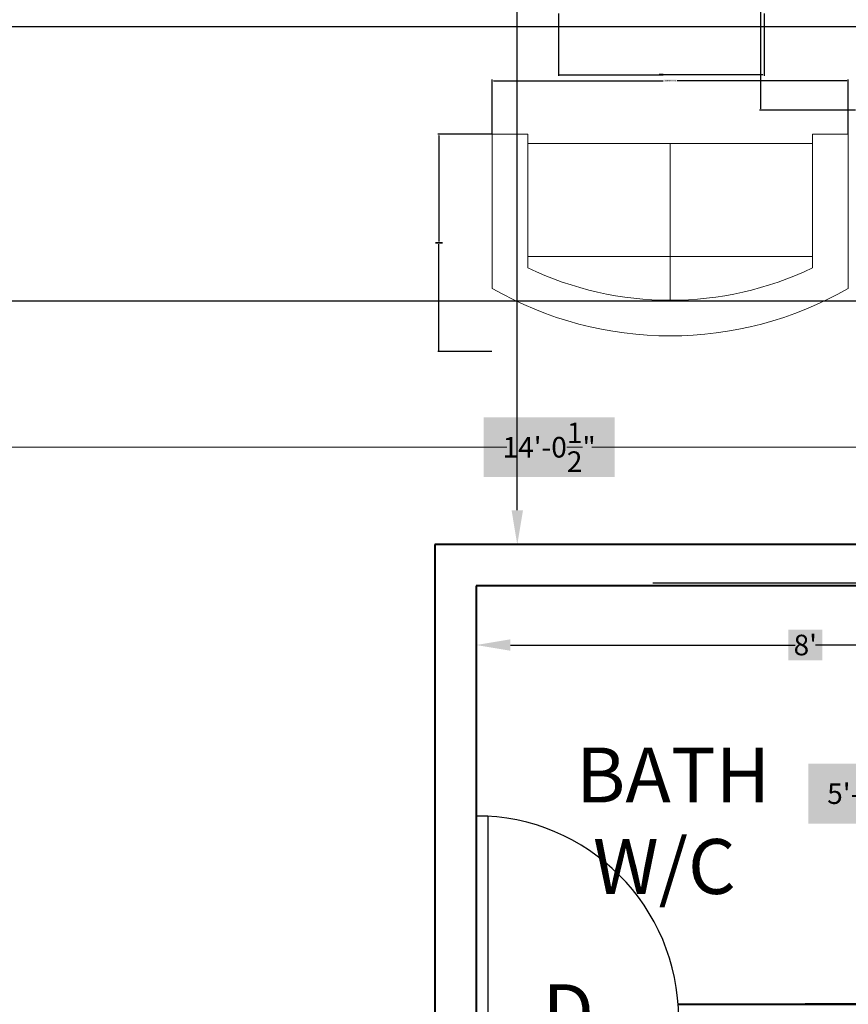
# Model space of a CAD drawing. Units: inches. Extents: x -301 to 715, y -607 to 364.
# Tile 97 of 141: x -39 to 82, y -77 to 67. Entities that reach past the tile are written whole.
import ezdxf

# ---------------------------------------------------------------- set-up
doc = ezdxf.new("R2010")
doc.units = ezdxf.units.IN
doc.header["$MEASUREMENT"] = 0
for name, color, linetype, lineweight in [('A-ANNO-DIMS', 2, 'Continuous', 18), ('A-ANNO-TEXT', 4, 'Continuous', 18), ('A-AREA-IDEN', 220, 'Continuous', 25), ('A-DOOR', 4, 'Continuous', 25), ('A-FURN', 8, 'Continuous', 18), ('A-WALL', 3, 'Continuous', 40)]:
    doc.layers.add(name, color=color, linetype=linetype, lineweight=lineweight)
doc.styles.get("Standard").update_dxf_attribs({"font": 'arial.ttf'})
doc.dimstyles.get("Standard").update_dxf_attribs({"dimtxt": 0.18, "dimasz": 0.18, "dimexe": 0.18, "dimexo": 0.0625, "dimgap": 0.09, "dimtad": 0, "dimtih": 1, "dimtoh": 1, "dimdec": 1, "dimzin": 0, "dimdsep": 46, "dimlunit": 4, "dimtxsty": 'Standard', "dimcen": 0.09, "dimclrd": 3, "dimclre": 4, "dimclrt": 6, "dimadec": 0, "dimazin": 0, "dimtfac": 1, "dimtdec": 1, "dimtofl": 0, "dimtmove": 0, "dimatfit": 3, "dimfxl": 1, "dimtfill": 2, "dimtfillclr": 51, "dimtolj": 1, "dimtzin": 0, "dimarcsym": 0})

# ---------------------------------------------------------------- blocks, each defined once
blk = doc.blocks.new('*U2')
for p, q in [((0, 0), (0, -100)), ((750, 0), (750, -100))]:
    blk.add_line(p, q)
blk.add_lwpolyline([(0, 0), (0, 750), (43.75, 750), (43.75, 0)], close=True)
blk.add_arc((0, 0), 750, 0, 90)
blk = doc.blocks.new('Sofa - Roundback Loveseat 5 ft.')
for p, q in [((0, -32.44198), (0, -5.99998)), ((-24, -33.99998), (-24, -11.46958)), ((24.00004, -33.99998), (24.00004, -11.46958)), ((-23.9998, -13.38178), (23.99986, -13.38178)), ((-24, -32.44198), (24.00004, -32.44198))]:
    blk.add_line(p, q)
for points in [[(-24, -33.99998), (-30, -33.99998), (-30, -7.99998)], [(30.00004, -7.99998), (30.00004, -33.99998), (24.00004, -33.99998)]]:
    blk.add_lwpolyline(points)
for centre, radius, start, end in [((0, -60.24998), 60.24998, 60.13715, 119.8628), ((0, -61.38438), 55.38444, 64.32083, 115.6792)]:
    blk.add_arc(centre, radius, start, end)
blk = doc.blocks.new('*D46')
at = {"layer": 'A-ANNO-DIMS', "color": 0, "lineweight": -2, "transparency": 16777216}
for p, q in [((27.9, -15.88), (27.9, -24.64)), ((123.9, -15.88), (123.9, -24.64)), ((32.9, -24.46), (74.42, -24.46)), ((118.9, -24.46), (77.37, -24.46))]:
    blk.add_line(p, q, dxfattribs=at)
at = {"layer": 'A-ANNO-DIMS', "color": 0, "transparency": 16777216}
for points in [[(32.9, -23.63), (32.9, -25.29), (27.9, -24.46)], [(118.9, -23.63), (118.9, -25.29), (123.9, -24.46)]]:
    blk.add_solid(points, dxfattribs=at)
at = {"layer": 'Defpoints', "color": 0, "transparency": 16777216}
for p in [(27.9, -15.82), (123.9, -15.82), (123.9, -24.46)]:
    blk.add_point(p, dxfattribs=at)
at = {"layer": 'A-ANNO-DIMS', "color": 0, "transparency": 16777216, "insert": (75.9, -24.46), "char_height": 3, "attachment_point": 5, "bg_fill": 1, "box_fill_scale": 1.25, "bg_fill_color": 51, "bg_fill_transparency": 0}
blk.add_mtext("\\A1;8'", dxfattribs=at)
blk = doc.blocks.new('*D47')
at = {"layer": 'A-ANNO-DIMS', "color": 0, "lineweight": -2, "transparency": 16777216}
for p, q in [((53.67, -15.42), (84.93, -15.42)), ((84.75, -20.42), (84.75, -42.49)), ((84.75, -71.82), (84.75, -49.75)), ((57.41, -76.82), (84.93, -76.82))]:
    blk.add_line(p, q, dxfattribs=at)
at = {"layer": 'A-ANNO-DIMS', "color": 0, "transparency": 16777216}
for points in [[(83.92, -20.42), (85.59, -20.42), (84.75, -15.42)], [(83.92, -71.82), (85.59, -71.82), (84.75, -76.82)]]:
    blk.add_solid(points, dxfattribs=at)
at = {"layer": 'Defpoints', "color": 0, "transparency": 16777216}
for p in [(53.6, -15.42), (84.75, -15.42), (57.35, -76.82)]:
    blk.add_point(p, dxfattribs=at)
at = {"layer": 'A-ANNO-DIMS', "color": 0, "transparency": 16777216, "insert": (84.75, -46.12), "char_height": 3, "attachment_point": 5, "bg_fill": 1, "box_fill_scale": 1.25, "bg_fill_color": 51, "bg_fill_transparency": 0}
blk.add_mtext('\\A1;5\'-1{\\H1x;\\S1/2;}"', dxfattribs=at)
blk = doc.blocks.new('*D48')
at = {"layer": 'A-ANNO-DIMS', "color": 0, "lineweight": -2, "transparency": 16777216}
for p, q in [((-45.6, -7.66), (-45.6, 4.54)), ((122.71, -8.55), (122.71, 4.54))]:
    blk.add_line(p, q, dxfattribs=at)
at = {"layer": 'A-ANNO-DIMS', "color": 0, "lineweight": 0, "transparency": 16777216}
for p, q in [((-40.6, 4.36), (32.36, 4.36)), ((117.71, 4.36), (44.75, 4.36))]:
    blk.add_line(p, q, dxfattribs=at)
at = {"layer": 'A-ANNO-DIMS', "color": 0, "transparency": 16777216}
for points in [[(-40.6, 5.2), (-40.6, 3.53), (-45.6, 4.36)], [(117.71, 5.2), (117.71, 3.53), (122.71, 4.36)]]:
    blk.add_solid(points, dxfattribs=at)
at = {"layer": 'Defpoints', "color": 0, "transparency": 16777216}
for p in [(-45.6, 4.36), (-45.6, -7.72), (122.71, -8.61)]:
    blk.add_point(p, dxfattribs=at)
at = {"layer": 'A-ANNO-DIMS', "color": 0, "transparency": 16777216, "insert": (38.55, 4.36), "char_height": 3, "attachment_point": 5, "bg_fill": 1, "box_fill_scale": 1.25, "bg_fill_color": 51, "bg_fill_transparency": 0}
blk.add_mtext('\\A1;14\'-0{\\H1x;\\S1/2;}"', dxfattribs=at)
blk = doc.blocks.new('*D49')
at = {"layer": 'A-ANNO-DIMS', "color": 0, "lineweight": -2, "transparency": 16777216}
for p, q in [((15.96, 193.18), (34.08, 193.18)), ((33.9, 188.18), (33.9, 93.3)), ((33.9, -4.82), (33.9, 90.06)), ((21.96, -9.82), (34.08, -9.82))]:
    blk.add_line(p, q, dxfattribs=at)
at = {"layer": 'A-ANNO-DIMS', "color": 0, "transparency": 16777216}
for points in [[(33.07, 188.18), (34.74, 188.18), (33.9, 193.18)], [(33.07, -4.82), (34.74, -4.82), (33.9, -9.82)]]:
    blk.add_solid(points, dxfattribs=at)
at = {"layer": 'Defpoints', "color": 0, "transparency": 16777216}
for p in [(15.9, 193.18), (33.9, 193.18), (21.9, -9.82)]:
    blk.add_point(p, dxfattribs=at)
at = {"layer": 'A-ANNO-DIMS', "color": 0, "transparency": 16777216, "insert": (33.9, 91.68), "char_height": 3, "attachment_point": 5, "bg_fill": 1, "box_fill_scale": 1.25, "bg_fill_color": 51, "bg_fill_transparency": 0}
blk.add_mtext('\\A1;16\'-11"', dxfattribs=at)
blk = doc.blocks.new('*D131')
at = {"layer": 'A-ANNO-DIMS', "color": 4, "lineweight": -2, "transparency": 16777216}
for p, q in [((39.9, 67.59), (39.9, 58.47)), ((69.9, 67.59), (69.9, 58.47))]:
    blk.add_line(p, q, dxfattribs=at)
at = {"layer": 'A-ANNO-DIMS', "color": 3, "lineweight": -2, "transparency": 16777216}
for p, q in [((40.08, 58.65), (54.57, 58.65)), ((69.72, 58.65), (55.23, 58.65))]:
    blk.add_line(p, q, dxfattribs=at)
at = {"layer": 'A-ANNO-DIMS', "color": 3, "transparency": 16777216}
for points in [[(40.08, 58.68), (40.08, 58.62), (39.9, 58.65)], [(69.72, 58.68), (69.72, 58.62), (69.9, 58.65)]]:
    blk.add_solid(points, dxfattribs=at)
at = {"layer": 'Defpoints', "color": 0, "transparency": 16777216}
for p in [(39.9, 67.65), (69.9, 67.65), (39.9, 58.65)]:
    blk.add_point(p, dxfattribs=at)
at = {"layer": 'A-ANNO-DIMS', "color": 6, "transparency": 16777216, "insert": (54.9, 58.65), "char_height": 0.18, "attachment_point": 5, "bg_fill": 1, "box_fill_scale": 1.25, "bg_fill_color": 51, "bg_fill_transparency": 0}
blk.add_mtext('\\A1;2\'-6"', dxfattribs=at)
blk = doc.blocks.new('*D132')
at = {"layer": 'A-ANNO-DIMS', "color": 4, "lineweight": -2, "transparency": 16777216}
for p, q in [((83.22, 145.95), (69.24, 145.95)), ((83.22, 53.5), (69.24, 53.5))]:
    blk.add_line(p, q, dxfattribs=at)
at = {"layer": 'A-ANNO-DIMS', "color": 3, "lineweight": -2, "transparency": 16777216}
for p, q in [((69.42, 145.77), (69.42, 99.91)), ((69.42, 53.68), (69.42, 99.55))]:
    blk.add_line(p, q, dxfattribs=at)
at = {"layer": 'A-ANNO-DIMS', "color": 3, "transparency": 16777216}
for points in [[(69.39, 145.77), (69.45, 145.77), (69.42, 145.95)], [(69.39, 53.68), (69.45, 53.68), (69.42, 53.5)]]:
    blk.add_solid(points, dxfattribs=at)
at = {"layer": 'Defpoints', "color": 0, "transparency": 16777216}
for p in [(83.29, 145.95), (69.42, 53.5), (83.29, 53.5)]:
    blk.add_point(p, dxfattribs=at)
at = {"layer": 'A-ANNO-DIMS', "color": 6, "transparency": 16777216, "insert": (69.42, 99.73), "char_height": 0.18, "attachment_point": 5, "bg_fill": 1, "box_fill_scale": 1.25, "bg_fill_color": 51, "bg_fill_transparency": 0}
blk.add_mtext('\\A1;SOFA 7\'-8 1/2"', dxfattribs=at)
blk = doc.blocks.new('*D134')
at = {"layer": 'A-ANNO-DIMS', "color": 4, "lineweight": -2, "transparency": 16777216}
for p, q in [((30.26, 50.05), (30.26, 57.95)), ((82.14, 50.05), (82.14, 57.95))]:
    blk.add_line(p, q, dxfattribs=at)
at = {"layer": 'A-ANNO-DIMS', "color": 3, "lineweight": -2, "transparency": 16777216}
for p, q in [((30.44, 57.77), (55.18, 57.77)), ((81.96, 57.77), (57.22, 57.77))]:
    blk.add_line(p, q, dxfattribs=at)
at = {"layer": 'A-ANNO-DIMS', "color": 3, "transparency": 16777216}
for points in [[(30.44, 57.8), (30.44, 57.74), (30.26, 57.77)], [(81.96, 57.8), (81.96, 57.74), (82.14, 57.77)]]:
    blk.add_solid(points, dxfattribs=at)
at = {"layer": 'Defpoints', "color": 0, "transparency": 16777216}
for p in [(30.26, 57.77), (30.26, 49.99), (82.14, 49.99)]:
    blk.add_point(p, dxfattribs=at)
at = {"layer": 'A-ANNO-DIMS', "color": 6, "transparency": 16777216, "insert": (56.2, 57.77), "char_height": 0.18, "attachment_point": 5, "bg_fill": 1, "box_fill_scale": 1.25, "bg_fill_color": 51, "bg_fill_transparency": 0}
blk.add_mtext('\\A1;LOVESEAT 4\'-4"', dxfattribs=at)
blk = doc.blocks.new('*D135')
at = {"layer": 'A-ANNO-DIMS', "color": 4, "lineweight": -2, "transparency": 16777216}
for p, q in [((30.2, 49.99), (22.3, 49.99)), ((30.2, 18.29), (22.3, 18.29))]:
    blk.add_line(p, q, dxfattribs=at)
at = {"layer": 'A-ANNO-DIMS', "color": 3, "lineweight": -2, "transparency": 16777216}
for p, q in [((22.48, 49.81), (22.48, 34.32)), ((22.48, 18.47), (22.48, 33.96))]:
    blk.add_line(p, q, dxfattribs=at)
at = {"layer": 'A-ANNO-DIMS', "color": 3, "transparency": 16777216}
for points in [[(22.45, 49.81), (22.51, 49.81), (22.48, 49.99)], [(22.45, 18.47), (22.51, 18.47), (22.48, 18.29)]]:
    blk.add_solid(points, dxfattribs=at)
at = {"layer": 'Defpoints', "color": 0, "transparency": 16777216}
for p in [(30.26, 49.99), (22.48, 18.29), (30.26, 18.29)]:
    blk.add_point(p, dxfattribs=at)
at = {"layer": 'A-ANNO-DIMS', "color": 6, "transparency": 16777216, "insert": (22.48, 34.14), "char_height": 0.18, "attachment_point": 5, "bg_fill": 1, "box_fill_scale": 1.25, "bg_fill_color": 51, "bg_fill_transparency": 0}
blk.add_mtext('\\A1;2\'-7 1/2"', dxfattribs=at)
blk = doc.blocks.new('*D149')
at = {"layer": 'A-ANNO-DIMS', "color": 4, "lineweight": -2, "transparency": 16777216}
for p, q in [((-51.54, 65.68), (233.66, 65.68)), ((-51.54, 25.68), (233.66, 25.68))]:
    blk.add_line(p, q, dxfattribs=at)
at = {"layer": 'A-ANNO-DIMS', "color": 3, "lineweight": -2, "transparency": 16777216}
for p, q in [((233.48, 65.5), (233.48, 45.86)), ((233.48, 25.86), (233.48, 45.5))]:
    blk.add_line(p, q, dxfattribs=at)
at = {"layer": 'A-ANNO-DIMS', "color": 3, "transparency": 16777216}
for points in [[(233.45, 65.5), (233.51, 65.5), (233.48, 65.68)], [(233.45, 25.86), (233.51, 25.86), (233.48, 25.68)]]:
    blk.add_solid(points, dxfattribs=at)
at = {"layer": 'Defpoints', "color": 0, "transparency": 16777216}
for p in [(-51.6, 65.68), (-51.6, 25.68), (233.48, 25.68)]:
    blk.add_point(p, dxfattribs=at)
at = {"layer": 'A-ANNO-DIMS', "color": 6, "transparency": 16777216, "insert": (233.48, 45.68), "char_height": 0.18, "attachment_point": 5, "bg_fill": 1, "box_fill_scale": 1.25, "bg_fill_color": 51, "bg_fill_transparency": 0}
blk.add_mtext('\\A1;3\'-4"', dxfattribs=at)

msp = doc.modelspace()

# ---------------------------------------------------------------- linework, layer by layer
at = {"layer": 'A-WALL'}
for p, q in [((21.9, -9.82), (21.9, -82.82)), ((123.9, -9.82), (21.9, -9.82)), ((123.9, -15.82), (27.9, -15.82)), ((27.9, -15.82), (27.9, -82.82)), ((57.35, -76.82), (123.9, -76.82)), ((123.9, -76.82), (75.9, -76.82))]:
    msp.add_line(p, q, dxfattribs=at)

# ---------------------------------------------------------------- block references
at = {"layer": 'A-DOOR', "xscale": 0.0393700787401575, "yscale": 0.0393700787401575, "zscale": 0.0393700787401575}
msp.add_blockref('*U2', (27.9, -78.88), dxfattribs=at)
at = {"layer": 'A-FURN', "xscale": 0.8646946346220261, "yscale": 0.8646946346220261, "zscale": 0.8646946346220261, "rotation": 180}
msp.add_blockref('Sofa - Roundback Loveseat 5 ft.', (56.2, 20.59), dxfattribs=at)

# ---------------------------------------------------------------- texts
at = {"layer": 'A-ANNO-TEXT'}
msp.add_text('D', height=8, dxfattribs=at).set_placement((37.58, -81.89))
at = {"layer": 'A-AREA-IDEN', "insert": (42.49, -39.4), "char_height": 8, "attachment_point": 1}
msp.add_mtext_dynamic_manual_height_columns('BATH\\P W/C', width=73.06, gutter_width=1, heights=[0], dxfattribs=at)

# ---------------------------------------------------------------- dimensions: what is measured, and where the dimension line sits
at = {"layer": 'A-ANNO-DIMS'}
for base, p1, p2, angle, override, picture, middle in [((33.9, 193.18), (21.9, -9.82), (15.9, 193.18), 90, {"dimtxt": 3, "dimasz": 5, "dimclrd": 0, "dimclre": 0, "dimclrt": 0}, '*D49', (33.9, 91.68)), ((39.9, 58.65), (69.9, 67.65), (39.9, 67.65), 180, {"dimdec": 1, "dimlfac": 1, "dimrnd": 0, "dimzin": 1, "dimdsep": 46, "dimlunit": 4, "dimfrac": 2}, '*D131', (54.9, 58.65)), ((233.48, 25.68), (-51.6, 65.68), (-51.6, 25.68), 90, {"dimdec": 1, "dimlfac": 1, "dimrnd": 0, "dimzin": 1, "dimdsep": 46, "dimlunit": 4, "dimfrac": 2}, '*D149', (233.48, 45.68)), ((22.48, 18.29), (30.26, 49.99), (30.26, 18.29), 270, {"dimdec": 1, "dimlfac": 1, "dimrnd": 0, "dimzin": 1, "dimdsep": 46, "dimlunit": 4, "dimfrac": 2}, '*D135', (22.48, 34.14)), ((84.75, -15.42), (57.35, -76.82), (53.6, -15.42), 90, {"dimtxt": 3, "dimasz": 5, "dimclrd": 0, "dimclre": 0, "dimclrt": 0}, '*D47', (84.75, -46.12))]:
    dim = msp.add_linear_dim(base=base, p1=p1, p2=p2, angle=angle, dimstyle='Standard', override=override, dxfattribs=at)
    dim.commit()
    dim.dimension.update_dxf_attribs({"geometry": picture, "text_midpoint": middle})
for base, p1, p2, angle, text, picture, middle in [((69.4192, 53.5044), (83.2867, 145.9543), (83.2867, 53.5044), 270, 'SOFA <>', '*D132', (69.4192, 99.7293)), ((30.26, 57.77), (82.14, 49.99), (30.26, 49.99), 180, 'LOVESEAT <>', '*D134', (56.2, 57.77))]:
    dim = msp.add_linear_dim(base=base, p1=p1, p2=p2, angle=angle, text=text, dimstyle='Standard', override={"dimdec": 1, "dimlfac": 1, "dimrnd": 0, "dimzin": 1, "dimdsep": 46, "dimlunit": 4, "dimfrac": 2}, dxfattribs=at)
    dim.commit()
    dim.dimension.update_dxf_attribs({"geometry": picture, "text_midpoint": middle})
for base, p1, p2, override, picture, middle in [((-45.6, 4.36), (122.71, -8.61), (-45.6, -7.72), {"dimtxt": 3, "dimasz": 5, "dimclrd": 0, "dimclre": 0, "dimclrt": 0, "dimlwd": 0}, '*D48', (38.55, 4.36)), ((123.9, -24.46), (27.9, -15.82), (123.9, -15.82), {"dimtxt": 3, "dimasz": 5, "dimclrd": 0, "dimclre": 0, "dimclrt": 0}, '*D46', (75.9, -24.46))]:
    dim = msp.add_linear_dim(base=base, p1=p1, p2=p2, dimstyle='Standard', override=override, dxfattribs=at)
    dim.commit()
    dim.dimension.update_dxf_attribs({"geometry": picture, "text_midpoint": middle})

doc.saveas('drawing.dxf')
